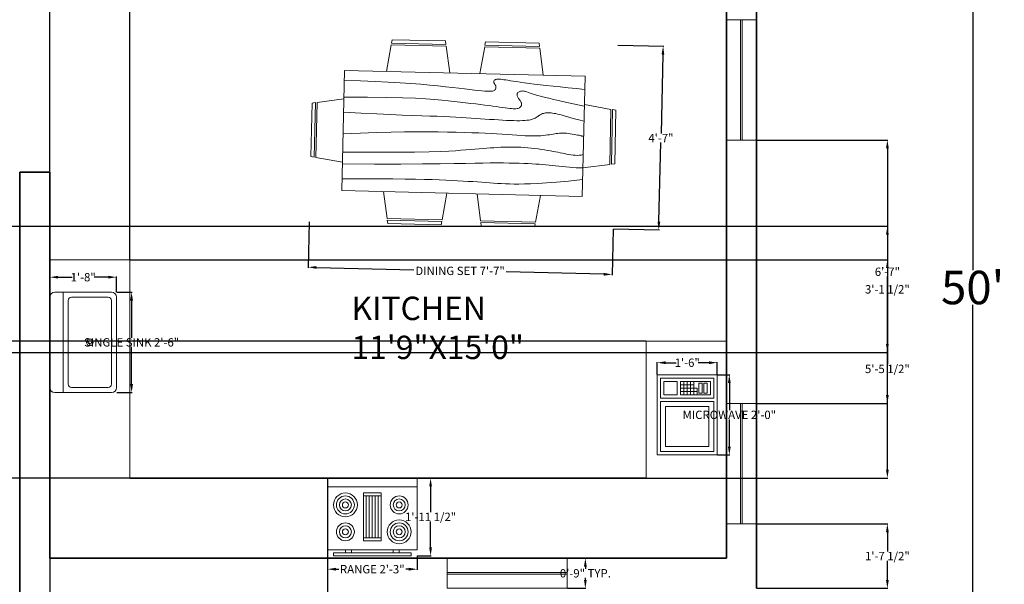
# Model space of a CAD drawing. Units: inches. Extents: x 481 to 2783, y 1975 to 3327.
# Tile 8 of 13: x 1574 to 1869, y 2866 to 3034. Entities that reach past the tile are written whole.
import ezdxf

# ---------------------------------------------------------------- set-up
doc = ezdxf.new("R2010")
doc.units = ezdxf.units.IN
doc.header["$MEASUREMENT"] = 0
for name, color, linetype, lineweight in [('A-ANNO-DIMS', 50, 'Continuous', 18), ('A-AREA-IDEN', 50, 'Continuous', 18), ('A-FLOR-CASE', 61, 'Continuous', 18), ('A-FLOR-FIXT', 61, 'Continuous', 18), ('A-FURN', 61, 'Continuous', 18), ('A-WALL', 40, 'Continuous', 35), ('EQUIPMENTS', 61, 'Continuous', 18), ('WINDOWS', 220, 'Continuous', 20)]:
    doc.layers.add(name, color=color, linetype=linetype, lineweight=lineweight)
doc.styles.get("Standard").update_dxf_attribs({"font": 'arial.ttf'})
doc.dimstyles.get("Standard").update_dxf_attribs({"dimtxt": 2.5, "dimasz": 2.5, "dimexe": 0.18, "dimexo": 0.0625, "dimgap": 0.09, "dimtad": 0, "dimtih": 1, "dimtoh": 1, "dimzin": 0, "dimdsep": 46, "dimlunit": 3, "dimtxsty": 'Standard', "dimcen": 0.09, "dimadec": 0, "dimazin": 0, "dimtfac": 1, "dimtofl": 0, "dimtmove": 0, "dimatfit": 3, "dimfxl": 1, "dimtolj": 1, "dimtzin": 0, "dimarcsym": 0})

# ---------------------------------------------------------------- blocks, each defined once
blk = doc.blocks.new('Microwave')
for p, q in [((18, 10), (22, 10)), ((22, 9), (18, 9)), ((19, 7), (19, 11)), ((20, 11), (20, 7)), ((21, 7), (21, 11)), ((18, 8), (22, 8)), ((22, 7), (18, 7)), ((20, 6), (18, 6)), ((19, 6), (19, 7)), ((20, 7), (20, 6))]:
    blk.add_line(p, q)
for points in [[(0, 0), (0, 18), (24, 18), (24, 0)], [(1, 1), (1, 17), (16, 17), (16, 1)], [(2.5, 2.5), (2.5, 15.5), (14.5, 15.5), (14.5, 2.5)], [(17, 1), (17, 17), (23, 17), (23, 1)], [(18, 12), (18, 16), (22, 16), (22, 12)], [(18, 2), (18, 11), (22, 11), (22, 2)], [(18.5, 4.5), (18.5, 5.5), (21.5, 5.5), (21.5, 4.5)], [(18.5, 3), (18.5, 4), (21.5, 4), (21.5, 3)]]:
    blk.add_lwpolyline(points, close=True)
blk = doc.blocks.new('Sink-single - 30 in top')
blk.add_line((-15, -3.999996), (15, -3.999996))
for points in [[(-13.5, 0), (13.5, 0)], [(-15, -18.499996), (-15, -1.5)], [(15, -1.5), (15, -18.499996)], [(-12.5, -5.499996), (12.5, -5.499996)], [(-13.5, -17.499996), (-13.5, -6.499996)], [(13.5, -6.499996), (13.5, -17.499996)], [(13.5, -19.999996), (-13.5, -19.999996)], [(12.5, -18.499996), (-12.5, -18.499996)]]:
    blk.add_lwpolyline(points)
for radius in [1, 0.5]:
    blk.add_circle((0, -11.999996), radius)
for centre, radius, start, end in [((-13.5, -1.5), 1.5, 90, 180), ((13.5, -1.5), 1.5, 0, 90), ((-12.5, -6.499996), 1, 90, 180), ((12.5, -6.499996), 1, 0, 90), ((-12.5, -17.499996), 1, 180, 270), ((12.5, -17.499996), 1, 270, 0), ((-13.5, -18.499996), 1.5, 180, 270), ((13.5, -18.499996), 1.5, 270, 0)]:
    blk.add_arc(centre, radius, start, end)
blk = doc.blocks.new('Dining Set - 36 x 72 in.')
for p, q in [((-22, 27.5), (-22.1562, 26.50042)), ((-22, 27.5), (-6, 27.5)), ((-5.8437, 26.49966), (-6, 27.5)), ((6, 27.5), (5.8438, 26.50042)), ((6, 27.5), (22, 27.5)), ((22.1563, 26.49966), (22, 27.5)), ((-22.2343, 26.00059), (-23.4847, 17.99762)), ((-22.2304, 26), (-5.7608, 26)), ((-5.8416, 26.5), (-22.1534, 26.5)), ((-4.5152, 17.99762), (-5.7655, 25.99926)), ((5.7657, 26.00059), (4.5153, 17.99762)), ((5.7696, 26), (22.2392, 26)), ((22.1584, 26.5), (5.8466, 26.5)), ((23.4848, 17.99762), (22.2345, 25.99926)), ((36, 18), (-36, 18)), ((-36, 18), (-36, -18)), ((36, -18), (36, 18)), ((-44.0006, 8.23428), (-35.9976, 9.48474)), ((44.0006, 8.23428), (35.9976, 9.48474)), ((-45.5, 8), (-44.5004, 8.15617)), ((-45.5, 8), (-45.5, -8)), ((-44.5, -8.15843), (-44.5, 8.15338)), ((-44, 8.23041), (-44, -8.23915)), ((44, 8.23041), (44, -8.23915)), ((44.5, -8.15843), (44.5, 8.15338)), ((45.5, 8), (44.5005, 8.15617)), ((45.5, 8), (45.5, -8)), ((-44.4997, -8.15631), (-45.5, -8)), ((-35.9976, -9.48476), (-43.9993, -8.2345)), ((35.9976, -9.48476), (43.9993, -8.2345)), ((44.4997, -8.15631), (45.5, -8)), ((-36, -18), (36, -18)), ((-22.2343, -26.0006), (-23.4847, -17.99762)), ((-4.5152, -17.99762), (-5.7655, -25.99928)), ((5.7657, -26.0006), (4.5153, -17.99762)), ((23.4848, -17.99762), (22.2345, -25.99928)), ((-22.2304, -26), (-5.7608, -26)), ((-22, -27.5), (-22.1562, -26.50044)), ((-5.8416, -26.5), (-22.1534, -26.5)), ((-5.8437, -26.49967), (-6, -27.5)), ((5.7696, -26), (22.2392, -26)), ((6, -27.5), (5.8438, -26.50044)), ((22.1584, -26.5), (5.8466, -26.5)), ((22.1563, -26.49967), (22, -27.5)), ((-22, -27.5), (-6, -27.5)), ((6, -27.5), (22, -27.5))]:
    blk.add_line(p, q)
for points in [[(-36, 15), (-31.1772, 14.97754), (-26.8079, 14.91406), (-22.8538, 14.81543), (-19.276, 14.6875), (-16.0362, 14.53613), (-13.0957, 14.36718), (-10.4159, 14.18652), (-7.9583, 14), (-5.6904, 13.81315), (-3.6035, 13.63021), (-1.6954, 13.45508), (0.0365, 13.29166), (1.5945, 13.14388), (2.9811, 13.01562), (4.1988, 12.9108), (5.25, 12.83333), (6.1393, 12.78613), (6.8802, 12.76823), (7.4883, 12.77767), (7.9792, 12.8125), (8.3685, 12.87077), (8.6719, 12.95052), (8.9049, 13.0498), (9.0833, 13.16666), (9.2205, 13.29899), (9.3216, 13.44401), (9.3895, 13.59879), (9.4271, 13.76041), (9.4373, 13.92594), (9.4232, 14.09245), (9.3875, 14.257), (9.3333, 14.41666), (9.2638, 14.56917), (9.1836, 14.71484), (9.0975, 14.85465), (9.0104, 14.98958), (8.9272, 15.1206), (8.8529, 15.2487), (8.7922, 15.37483), (8.75, 15.5), (8.7305, 15.62467), (8.7344, 15.74739), (8.7617, 15.86621), (8.8125, 15.97916), (8.8867, 16.08431), (8.9844, 16.17968), (9.1055, 16.26334), (9.25, 16.33333), (9.4189, 16.38802), (9.6172, 16.42708), (9.8506, 16.45052), (10.125, 16.45833), (10.4463, 16.45052), (10.8203, 16.42708), (11.2529, 16.38802), (11.75, 16.33333), (12.3184, 16.26318), (12.9694, 16.17838), (13.7151, 16.07991), (14.5677, 15.96875), (15.5395, 15.84586), (16.6426, 15.71224), (17.8893, 15.56884), (19.2917, 15.41666), (20.859, 15.25667), (22.5879, 15.08984), (24.4721, 14.91715), (26.5052, 14.73958), (28.6809, 14.5581), (30.9929, 14.3737), (33.4347, 14.18733), (36, 14)], [(-36, 10), (-28.9766, 10.14274), (-23.1725, 10.20442), (-18.4241, 10.19775), (-14.5677, 10.13541), (-11.4399, 10.03011), (-8.877, 9.89453), (-6.7154, 9.74137), (-4.7917, 9.58333), (-2.9698, 9.43082), (-1.2246, 9.28515), (0.4415, 9.14534), (2.026, 9.01041), (3.5266, 8.87939), (4.9408, 8.7513), (6.266, 8.62516), (7.5, 8.5), (8.6411, 8.37549), (9.6914, 8.2539), (10.6538, 8.13818), (11.5312, 8.03125), (12.3267, 7.93603), (13.043, 7.85547), (13.6831, 7.79248), (14.25, 7.75), (14.7471, 7.7303), (15.1797, 7.73307), (15.5537, 7.75732), (15.875, 7.80208), (16.1494, 7.86637), (16.3828, 7.94922), (16.5811, 8.04964), (16.75, 8.16666), (16.8944, 8.29915), (17.0143, 8.44531), (17.1089, 8.60319), (17.1771, 8.77083), (17.218, 8.94629), (17.2305, 9.1276), (17.2137, 9.31282), (17.1667, 9.5), (17.0895, 9.6875), (16.987, 9.875), (16.8649, 10.0625), (16.7292, 10.25), (16.5856, 10.4375), (16.4401, 10.625), (16.2985, 10.8125), (16.1667, 11), (16.05, 11.18733), (15.9518, 11.3737), (15.8752, 11.5581), (15.8229, 11.73958), (15.798, 11.91715), (15.8034, 12.08984), (15.842, 12.25667), (15.9167, 12.41666), (16.0295, 12.56836), (16.1784, 12.70833), (16.3605, 12.83268), (16.5729, 12.9375), (16.8127, 13.01888), (17.0768, 13.07291), (17.3625, 13.0957), (17.6667, 13.08333), (17.9894, 13.03312), (18.3418, 12.94726), (18.7382, 12.82918), (19.1927, 12.68229), (19.7195, 12.51001), (20.3327, 12.31575), (21.0465, 12.10294), (21.875, 11.875), (22.8357, 11.63354), (23.959, 11.37304), (25.2786, 11.08618), (26.8282, 10.76562), (28.6414, 10.40405), (30.752, 9.99414), (33.1936, 9.52856), (36, 9)], [(-36, 5.5), (-30.7157, 5.3348), (-26.069, 5.20963), (-21.9946, 5.11767), (-18.4271, 5.05208), (-15.3009, 5.00602), (-12.5508, 4.97265), (-10.1112, 4.94515), (-7.9167, 4.91666), (-5.909, 4.88167), (-4.0586, 4.83984), (-2.3429, 4.79215), (-0.7396, 4.73958), (0.7739, 4.6831), (2.22, 4.6237), (3.6213, 4.56233), (5, 4.5), (6.373, 4.43782), (7.7344, 4.3776), (9.0723, 4.32129), (10.375, 4.27083), (11.6309, 4.22819), (12.8281, 4.19531), (13.9551, 4.17415), (15, 4.16666), (15.954, 4.17448), (16.819, 4.19791), (17.6001, 4.23698), (18.3021, 4.29166), (18.9299, 4.36198), (19.4883, 4.44791), (19.9823, 4.54948), (20.4167, 4.66666), (20.7969, 4.79899), (21.1302, 4.94401), (21.4245, 5.09879), (21.6875, 5.26041), (21.9271, 5.42594), (22.1511, 5.59245), (22.3672, 5.757), (22.5834, 5.91666), (22.8065, 6.06868), (23.0404, 6.21093), (23.2879, 6.34147), (23.5521, 6.45833), (23.8358, 6.55957), (24.142, 6.64323), (24.4735, 6.70735), (24.8334, 6.75), (25.2235, 6.76969), (25.642, 6.76692), (26.0858, 6.74267), (26.5521, 6.69791), (27.0379, 6.63362), (27.5404, 6.55078), (28.0565, 6.45036), (28.5834, 6.33333), (29.1242, 6.19987), (29.7071, 6.04687), (30.3661, 5.87044), (31.1354, 5.66666), (32.0493, 5.43164), (33.142, 5.16146), (34.4475, 4.85221), (36, 4.5)], [(-36, -1), (-30.7915, -0.6591), (-26.0195, -0.38216), (-21.6519, -0.16284), (-17.6563, 0.00521), (-14.0005, 0.12833), (-10.6523, 0.21289), (-7.5796, 0.26522), (-4.75, 0.29166), (-2.134, 0.29793), (0.2878, 0.28711), (2.5317, 0.26163), (4.6146, 0.22396), (6.5529, 0.17651), (8.3633, 0.12174), (10.0623, 0.06209), (11.6667, 0), (13.1899, -0.06201), (14.6341, -0.1211), (15.9982, -0.17432), (17.2813, -0.21875), (18.4823, -0.25147), (19.6003, -0.26953), (20.6343, -0.27002), (21.5834, -0.25), (22.4481, -0.20768), (23.2357, -0.14584), (23.9549, -0.06836), (24.6146, 0.02083), (25.2235, 0.11784), (25.7904, 0.21875), (26.3241, 0.31966), (26.8334, 0.41666), (27.3265, 0.50618), (27.8099, 0.58593), (28.2894, 0.65397), (28.7709, 0.70833), (29.2601, 0.74707), (29.763, 0.76823), (30.2855, 0.76985), (30.8334, 0.75), (31.4088, 0.70784), (31.9994, 0.64713), (32.589, 0.57275), (33.1615, 0.48958), (33.7008, 0.4025), (34.1908, 0.3164), (34.6153, 0.23616), (34.9584, 0.16666), (35.2099, 0.11165), (35.3848, 0.07031), (35.504, 0.04069), (35.5886, 0.02083), (35.6594, 0.00879), (35.7377, 0.0026), (35.8442, 0.00032), (36, 0)], [(-36, -6.5), (-27.1843, -6.31267), (-20.084, -6.1263), (-14.469, -5.9419), (-10.1094, -5.76042), (-6.7752, -5.58285), (-4.2363, -5.41016), (-2.2629, -5.24333), (-0.625, -5.08334), (0.8708, -4.93099), (2.2715, -4.78646), (3.5872, -4.64974), (4.8281, -4.52084), (6.0046, -4.39974), (7.127, -4.28646), (8.2053, -4.18099), (9.25, -4.08334), (10.2705, -3.99382), (11.2734, -3.91407), (12.2647, -3.84603), (13.25, -3.79167), (14.2354, -3.75293), (15.2266, -3.73177), (16.2295, -3.73015), (17.25, -3.75), (18.2912, -3.79248), (19.3451, -3.85547), (20.4009, -3.93604), (21.4479, -4.03125), (22.4754, -4.13819), (23.4727, -4.25391), (24.4289, -4.37549), (25.3334, -4.5), (26.1785, -4.62492), (26.9694, -4.74935), (27.7145, -4.87281), (28.4219, -4.99479), (29.1, -5.11483), (29.7572, -5.23242), (30.4016, -5.34709), (31.0417, -5.45834), (31.6837, -5.56437), (32.3262, -5.65821), (32.9658, -5.73153), (33.599, -5.77604), (34.2224, -5.78345), (34.8327, -5.74545), (35.4264, -5.65373), (36, -5.5)], [(-36, -10), (-26.4022, -9.81299), (-18.4675, -9.62891), (-11.9839, -9.45069), (-6.7396, -9.28125), (-2.5226, -9.12354), (0.8789, -8.98047), (3.6769, -8.85498), (6.0833, -8.75), (8.2767, -8.66765), (10.3021, -8.60677), (12.1712, -8.56543), (13.8958, -8.54167), (15.4876, -8.53353), (16.9583, -8.53907), (18.3197, -8.55632), (19.5834, -8.58334), (20.7616, -8.61841), (21.8685, -8.66081), (22.9188, -8.71004), (23.9271, -8.76563), (24.9081, -8.82707), (25.8763, -8.89388), (26.8465, -8.96558), (27.8334, -9.04167), (28.8474, -9.12118), (29.8828, -9.20117), (30.93, -9.27824), (31.9792, -9.34896), (33.0205, -9.40991), (34.0443, -9.45768), (35.0407, -9.48885), (36, -9.5)], [(-36, -14.5), (-30.0881, -14.33513), (-25.0332, -14.21224), (-20.7312, -14.12647), (-17.0781, -14.07292), (-13.97, -14.04671), (-11.3027, -14.04297), (-8.9724, -14.05681), (-6.875, -14.08334), (-4.9224, -14.11833), (-3.0905, -14.16016), (-1.3709, -14.20785), (0.2448, -14.26042), (1.7647, -14.3169), (3.1973, -14.3763), (4.5507, -14.43767), (5.8333, -14.5), (7.0554, -14.5621), (8.235, -14.62175), (9.3922, -14.67652), (10.5469, -14.72396), (11.7192, -14.76164), (12.929, -14.78711), (14.1965, -14.79794), (15.5417, -14.79167), (16.9933, -14.76424), (18.6152, -14.70508), (20.4804, -14.60197), (22.6615, -14.44271), (25.2312, -14.21509), (28.2624, -13.9069), (31.8277, -13.50594), (36, -13)]]:
    blk.add_lwpolyline(points)
blk = doc.blocks.new('Range-Oven - 30 in top')
for p, q in [((0, -3), (30, -3)), ((12, -6), (18, -6)), ((13, -20), (13, -6)), ((14, -6), (14, -20)), ((15, -20), (15, -6)), ((16, -6), (16, -20)), ((17, -20), (17, -6)), ((18, -20), (12, -20)), ((6, -24), (6, -25)), ((8, -25), (8, -24)), ((22, -25), (22, -24)), ((24, -24), (24, -25))]:
    blk.add_line(p, q)
for points in [[(0, -24), (0, 0), (30, 0), (30, -24)], [(12, -21), (12, -5), (18, -5), (18, -21)], [(2, -26), (2, -25), (28, -25), (28, -26)]]:
    blk.add_lwpolyline(points, close=True)
for centre, radius in [((6, -9), 4), ((6, -9), 3), ((24, -9), 3), ((6, -9), 2), ((6, -9), 1), ((24, -9), 2), ((24, -9), 1), ((6, -18), 3), ((6, -18), 2), ((24, -18), 4), ((24, -18), 3), ((24, -18), 2), ((6, -18), 1), ((24, -18), 1)]:
    blk.add_circle(centre, radius)
blk = doc.blocks.new('*D23')
at = {"layer": 'A-ANNO-DIMS', "color": 0, "lineweight": -2, "transparency": 16777216}
for p, q in [((1794.5, 3254.32), (1859.35, 3254.32)), ((1859.17, 3249.32), (1859.17, 2959.52)), ((1859.17, 2659.32), (1859.17, 2949.13)), ((1794.5, 2654.32), (1859.35, 2654.32))]:
    blk.add_line(p, q, dxfattribs=at)
at = {"layer": 'A-ANNO-DIMS', "color": 0, "transparency": 16777216}
for points in [[(1858.33, 3249.32), (1860, 3249.32), (1859.17, 3254.32)], [(1858.33, 2659.32), (1860, 2659.32), (1859.17, 2654.32)]]:
    blk.add_solid(points, dxfattribs=at)
at = {"layer": 'Defpoints', "color": 0, "transparency": 16777216}
for p in [(1794.44, 3254.32), (1794.44, 2654.32), (1859.17, 2654.32)]:
    blk.add_point(p, dxfattribs=at)
at = {"layer": 'A-ANNO-DIMS', "color": 0, "transparency": 16777216, "insert": (1859.17, 2954.32), "char_height": 10, "attachment_point": 5}
blk.add_mtext("\\A1;50'", dxfattribs=at)
blk = doc.blocks.new('WIN-PLAN-36IN')
for p, q in [((0, 4.75), (36, 4.75)), ((0, 4.25), (36, 4.25))]:
    blk.add_line(p, q)
blk.add_lwpolyline([(0, 0), (36, 0), (36, 9), (0, 9)], close=True)
blk = doc.blocks.new('*D31')
at = {"layer": 'A-ANNO-DIMS', "color": 0, "lineweight": -2, "transparency": 16777216}
for p, q in [((1737.9, 2873.32), (1743.42, 2873.32)), ((1743.24, 2870.82), (1743.24, 2870.19)), ((1743.24, 2866.82), (1743.24, 2867.46)), ((1737.9, 2864.32), (1743.42, 2864.32))]:
    blk.add_line(p, q, dxfattribs=at)
at = {"layer": 'A-ANNO-DIMS', "color": 0, "transparency": 16777216}
for points in [[(1742.83, 2870.82), (1743.66, 2870.82), (1743.24, 2873.32)], [(1742.83, 2866.82), (1743.66, 2866.82), (1743.24, 2864.32)]]:
    blk.add_solid(points, dxfattribs=at)
at = {"layer": 'Defpoints', "color": 0, "transparency": 16777216}
for p in [(1737.84, 2873.32), (1743.24, 2873.32), (1737.84, 2864.32)]:
    blk.add_point(p, dxfattribs=at)
at = {"layer": 'A-ANNO-DIMS', "color": 0, "transparency": 16777216, "insert": (1743.24, 2868.82), "char_height": 2.5, "attachment_point": 5}
blk.add_mtext('\\A1;0\'-9" TYP.', dxfattribs=at)
blk = doc.blocks.new('*D38')
at = {"layer": 'A-ANNO-DIMS', "color": 0, "lineweight": -2, "transparency": 16777216}
for p, q in [((1782.8, 2928.23), (1786.52, 2928.23)), ((1786.34, 2925.73), (1786.34, 2917.61)), ((1786.34, 2906.73), (1786.34, 2914.84)), ((1782.8, 2904.23), (1786.52, 2904.23))]:
    blk.add_line(p, q, dxfattribs=at)
at = {"layer": 'A-ANNO-DIMS', "color": 0, "transparency": 16777216}
for points in [[(1785.92, 2925.73), (1786.76, 2925.73), (1786.34, 2928.23)], [(1785.92, 2906.73), (1786.76, 2906.73), (1786.34, 2904.23)]]:
    blk.add_solid(points, dxfattribs=at)
at = {"layer": 'Defpoints', "color": 0, "transparency": 16777216}
for p in [(1782.74, 2928.23), (1786.34, 2928.23), (1782.74, 2904.23)]:
    blk.add_point(p, dxfattribs=at)
at = {"layer": 'A-ANNO-DIMS', "color": 0, "transparency": 16777216, "insert": (1786.34, 2916.23), "char_height": 2.5, "attachment_point": 5}
blk.add_mtext('\\A1;MICROWAVE 2\'-0"', dxfattribs=at)
blk = doc.blocks.new('*D39')
at = {"layer": 'A-ANNO-DIMS', "color": 0, "lineweight": -2, "transparency": 16777216}
for p, q in [((1764.74, 2928.29), (1764.74, 2932.01)), ((1767.24, 2931.83), (1770.45, 2931.83)), ((1780.24, 2931.83), (1777.04, 2931.83)), ((1782.74, 2928.29), (1782.74, 2932.01))]:
    blk.add_line(p, q, dxfattribs=at)
at = {"layer": 'A-ANNO-DIMS', "color": 0, "transparency": 16777216}
for points in [[(1767.24, 2932.24), (1767.24, 2931.41), (1764.74, 2931.83)], [(1780.24, 2932.24), (1780.24, 2931.41), (1782.74, 2931.83)]]:
    blk.add_solid(points, dxfattribs=at)
at = {"layer": 'Defpoints', "color": 0, "transparency": 16777216}
for p in [(1764.74, 2931.83), (1764.74, 2928.23), (1782.74, 2928.23)]:
    blk.add_point(p, dxfattribs=at)
at = {"layer": 'A-ANNO-DIMS', "color": 0, "transparency": 16777216, "insert": (1773.74, 2931.83), "char_height": 2.5, "attachment_point": 5}
blk.add_mtext('\\A1;1\'-6"', dxfattribs=at)
blk = doc.blocks.new('*D42')
at = {"layer": 'A-ANNO-DIMS', "color": 0, "lineweight": -2, "transparency": 16777216}
for p, q in [((1603, 2952.91), (1607.62, 2952.91)), ((1607.44, 2950.41), (1607.44, 2939.29)), ((1607.44, 2925.41), (1607.44, 2936.53)), ((1603, 2922.91), (1607.62, 2922.91))]:
    blk.add_line(p, q, dxfattribs=at)
at = {"layer": 'A-ANNO-DIMS', "color": 0, "transparency": 16777216}
for points in [[(1607.02, 2950.41), (1607.85, 2950.41), (1607.44, 2952.91)], [(1607.02, 2925.41), (1607.85, 2925.41), (1607.44, 2922.91)]]:
    blk.add_solid(points, dxfattribs=at)
at = {"layer": 'Defpoints', "color": 0, "transparency": 16777216}
for p in [(1602.94, 2952.91), (1607.44, 2952.91), (1602.94, 2922.91)]:
    blk.add_point(p, dxfattribs=at)
at = {"layer": 'A-ANNO-DIMS', "color": 0, "transparency": 16777216, "insert": (1607.44, 2937.91), "char_height": 2.5, "attachment_point": 5}
blk.add_mtext('\\A1;SINGLE SINK 2\'-6"', dxfattribs=at)
blk = doc.blocks.new('*D43')
at = {"layer": 'A-ANNO-DIMS', "color": 0, "lineweight": -2, "transparency": 16777216}
for p, q in [((1582.94, 2952.97), (1582.94, 2957.59)), ((1585.44, 2957.41), (1589.64, 2957.41)), ((1600.44, 2957.41), (1596.23, 2957.41)), ((1602.94, 2952.97), (1602.94, 2957.59))]:
    blk.add_line(p, q, dxfattribs=at)
at = {"layer": 'A-ANNO-DIMS', "color": 0, "transparency": 16777216}
for points in [[(1585.44, 2957.83), (1585.44, 2956.99), (1582.94, 2957.41)], [(1600.44, 2957.83), (1600.44, 2956.99), (1602.94, 2957.41)]]:
    blk.add_solid(points, dxfattribs=at)
at = {"layer": 'Defpoints', "color": 0, "transparency": 16777216}
for p in [(1582.94, 2957.41), (1582.94, 2952.91), (1602.94, 2952.91)]:
    blk.add_point(p, dxfattribs=at)
at = {"layer": 'A-ANNO-DIMS', "color": 0, "transparency": 16777216, "insert": (1592.94, 2957.41), "char_height": 2.5, "attachment_point": 5}
blk.add_mtext('\\A1;1\'-8"', dxfattribs=at)
blk = doc.blocks.new('*D50')
at = {"layer": 'A-ANNO-DIMS', "color": 0, "lineweight": -2, "transparency": 16777216}
for p, q in [((1660.59, 2973.97), (1660.26, 2960.21)), ((1751.56, 2971.8), (1751.23, 2958.04)), ((1662.76, 2960.33), (1691.92, 2959.63)), ((1748.74, 2958.28), (1719.58, 2958.98))]:
    blk.add_line(p, q, dxfattribs=at)
at = {"layer": 'A-ANNO-DIMS', "color": 0, "transparency": 16777216}
for points in [[(1662.77, 2960.74), (1662.75, 2959.91), (1660.26, 2960.39)], [(1748.75, 2958.7), (1748.73, 2957.86), (1751.24, 2958.22)]]:
    blk.add_solid(points, dxfattribs=at)
at = {"layer": 'Defpoints', "color": 0, "transparency": 16777216}
for p in [(1660.59, 2974.03), (1751.56, 2971.87), (1751.24, 2958.22)]:
    blk.add_point(p, dxfattribs=at)
at = {"layer": 'A-ANNO-DIMS', "color": 0, "transparency": 16777216, "insert": (1705.75, 2959.3), "char_height": 2.5, "attachment_point": 5}
blk.add_mtext('\\A1;DINING SET 7\'-7"', dxfattribs=at)
blk = doc.blocks.new('*D51')
at = {"layer": 'A-ANNO-DIMS', "color": 0, "lineweight": -2, "transparency": 16777216}
for p, q in [((1752.93, 3026.85), (1766.7, 3026.52)), ((1766.46, 3024.03), (1765.89, 3000.37)), ((1765.27, 2974.04), (1765.83, 2997.69)), ((1751.62, 2971.87), (1765.39, 2971.54))]:
    blk.add_line(p, q, dxfattribs=at)
at = {"layer": 'A-ANNO-DIMS', "color": 0, "transparency": 16777216}
for points in [[(1766.04, 3024.04), (1766.87, 3024.02), (1766.52, 3026.53)], [(1764.85, 2974.05), (1765.68, 2974.03), (1765.21, 2971.54)]]:
    blk.add_solid(points, dxfattribs=at)
at = {"layer": 'Defpoints', "color": 0, "transparency": 16777216}
for p in [(1752.87, 3026.85), (1766.52, 3026.53), (1751.56, 2971.87)]:
    blk.add_point(p, dxfattribs=at)
at = {"layer": 'A-ANNO-DIMS', "color": 0, "transparency": 16777216, "insert": (1765.86, 2999.03), "char_height": 2.5, "attachment_point": 5}
blk.add_mtext('\\A1;4\'-7"', dxfattribs=at)
blk = doc.blocks.new('*D52')
at = {"layer": 'A-ANNO-DIMS', "color": 0, "lineweight": -2, "transparency": 16777216}
for p, q in [((1666.06, 2874.01), (1666.06, 2869.86)), ((1692.89, 2874.01), (1692.89, 2869.86)), ((1668.56, 2870.04), (1669.43, 2870.04)), ((1690.39, 2870.04), (1689.52, 2870.04))]:
    blk.add_line(p, q, dxfattribs=at)
at = {"layer": 'A-ANNO-DIMS', "color": 0, "transparency": 16777216}
for points in [[(1668.56, 2870.46), (1668.56, 2869.63), (1666.06, 2870.04)], [(1690.39, 2870.46), (1690.39, 2869.63), (1692.89, 2870.04)]]:
    blk.add_solid(points, dxfattribs=at)
at = {"layer": 'Defpoints', "color": 0, "transparency": 16777216}
for p in [(1666.06, 2874.07), (1692.89, 2874.07), (1692.89, 2870.04)]:
    blk.add_point(p, dxfattribs=at)
at = {"layer": 'A-ANNO-DIMS', "color": 0, "transparency": 16777216, "insert": (1679.47, 2870.04), "char_height": 2.5, "attachment_point": 5}
blk.add_mtext('\\A1;RANGE 2\'-3"', dxfattribs=at)
blk = doc.blocks.new('*D53')
at = {"layer": 'A-ANNO-DIMS', "color": 0, "lineweight": -2, "transparency": 16777216}
for p, q in [((1692.95, 2897.32), (1697.1, 2897.32)), ((1696.92, 2894.82), (1696.92, 2887.08)), ((1696.92, 2876.57), (1696.92, 2884.31)), ((1692.95, 2874.07), (1697.1, 2874.07))]:
    blk.add_line(p, q, dxfattribs=at)
at = {"layer": 'A-ANNO-DIMS', "color": 0, "transparency": 16777216}
for points in [[(1696.5, 2894.82), (1697.33, 2894.82), (1696.92, 2897.32)], [(1696.5, 2876.57), (1697.33, 2876.57), (1696.92, 2874.07)]]:
    blk.add_solid(points, dxfattribs=at)
at = {"layer": 'Defpoints', "color": 0, "transparency": 16777216}
for p in [(1692.89, 2897.32), (1696.92, 2897.32), (1692.89, 2874.07)]:
    blk.add_point(p, dxfattribs=at)
at = {"layer": 'A-ANNO-DIMS', "color": 0, "transparency": 16777216, "insert": (1696.92, 2885.7), "char_height": 2.5, "attachment_point": 5}
blk.add_mtext('\\A1;1\'-11 1/2"', dxfattribs=at)
blk = doc.blocks.new('*D88')
at = {"layer": 'A-ANNO-DIMS', "color": 0, "lineweight": -2, "transparency": 16777216}
for p, q in [((1794.5, 2883.62), (1833.82, 2883.62)), ((1833.64, 2881.12), (1833.64, 2875.35)), ((1833.64, 2866.82), (1833.64, 2872.59)), ((1794.5, 2864.32), (1833.82, 2864.32))]:
    blk.add_line(p, q, dxfattribs=at)
at = {"layer": 'A-ANNO-DIMS', "color": 0, "transparency": 16777216}
for points in [[(1833.22, 2881.12), (1834.05, 2881.12), (1833.64, 2883.62)], [(1833.22, 2866.82), (1834.05, 2866.82), (1833.64, 2864.32)]]:
    blk.add_solid(points, dxfattribs=at)
at = {"layer": 'Defpoints', "color": 0, "transparency": 16777216}
for p in [(1794.44, 2883.62), (1833.64, 2883.62), (1794.44, 2864.32)]:
    blk.add_point(p, dxfattribs=at)
at = {"layer": 'A-ANNO-DIMS', "color": 0, "transparency": 16777216, "insert": (1833.64, 2873.97), "char_height": 2.5, "attachment_point": 5}
blk.add_mtext('\\A1;1\'-7 1/2"', dxfattribs=at)
blk = doc.blocks.new('*D89')
at = {"layer": 'A-ANNO-DIMS', "color": 0, "lineweight": -2, "transparency": 16777216}
for p, q in [((1794.5, 2998.45), (1833.82, 2998.45)), ((1833.64, 2995.95), (1833.64, 2960.4)), ((1833.64, 2922.12), (1833.64, 2957.67)), ((1794.5, 2919.62), (1833.82, 2919.62))]:
    blk.add_line(p, q, dxfattribs=at)
at = {"layer": 'A-ANNO-DIMS', "color": 0, "transparency": 16777216}
for points in [[(1833.22, 2995.95), (1834.05, 2995.95), (1833.64, 2998.45)], [(1833.22, 2922.12), (1834.05, 2922.12), (1833.64, 2919.62)]]:
    blk.add_solid(points, dxfattribs=at)
at = {"layer": 'Defpoints', "color": 0, "transparency": 16777216}
for p in [(1794.44, 2998.45), (1833.64, 2998.45), (1794.44, 2919.62)]:
    blk.add_point(p, dxfattribs=at)
at = {"layer": 'A-ANNO-DIMS', "color": 0, "transparency": 16777216, "insert": (1833.64, 2959.03), "char_height": 2.5, "attachment_point": 5}
blk.add_mtext('\\A1;6\'-7"', dxfattribs=at)
blk = doc.blocks.new('*D97')
at = {"layer": 'A-ANNO-DIMS', "color": 0, "lineweight": -2, "transparency": 16777216}
for p, q in [((1520, 2972.64), (1833.82, 2972.64)), ((1833.64, 2970.14), (1833.64, 2955.16)), ((1833.64, 2937.42), (1833.64, 2952.39)), ((1520, 2934.92), (1833.82, 2934.92))]:
    blk.add_line(p, q, dxfattribs=at)
at = {"layer": 'A-ANNO-DIMS', "color": 0, "transparency": 16777216}
for points in [[(1833.22, 2970.14), (1834.05, 2970.14), (1833.64, 2972.64)], [(1833.22, 2937.42), (1834.05, 2937.42), (1833.64, 2934.92)]]:
    blk.add_solid(points, dxfattribs=at)
at = {"layer": 'Defpoints', "color": 0, "transparency": 16777216}
for p in [(1519.94, 2972.64), (1833.64, 2972.64), (1519.94, 2934.92)]:
    blk.add_point(p, dxfattribs=at)
at = {"layer": 'A-ANNO-DIMS', "color": 0, "transparency": 16777216, "insert": (1833.64, 2953.78), "char_height": 2.5, "attachment_point": 5}
blk.add_mtext('\\A1;3\'-1 1/2"', dxfattribs=at)
blk = doc.blocks.new('*D101')
at = {"layer": 'A-ANNO-DIMS', "color": 0, "lineweight": -2, "transparency": 16777216}
for p, q in [((1582.94, 2962.67), (1582.94, 3293.7)), ((1585.44, 3293.52), (1591.5, 3293.52)), ((1604.44, 3293.52), (1598.37, 3293.52)), ((1606.94, 2962.67), (1606.94, 3293.7))]:
    blk.add_line(p, q, dxfattribs=at)
at = {"layer": 'A-ANNO-DIMS', "color": 0, "transparency": 16777216}
for points in [[(1585.44, 3293.94), (1585.44, 3293.11), (1582.94, 3293.52)], [(1604.44, 3293.94), (1604.44, 3293.11), (1606.94, 3293.52)]]:
    blk.add_solid(points, dxfattribs=at)
at = {"layer": 'Defpoints', "color": 0, "transparency": 16777216}
for p in [(1606.94, 3293.52), (1582.94, 2962.61), (1606.94, 2962.61)]:
    blk.add_point(p, dxfattribs=at)
at = {"layer": 'A-ANNO-DIMS', "color": 0, "transparency": 16777216, "insert": (1594.94, 3293.52), "char_height": 2.5, "attachment_point": 5}
blk.add_mtext('\\A1;2\'-0"', dxfattribs=at)
blk = doc.blocks.new('*D102')
at = {"layer": 'A-ANNO-DIMS', "color": 0, "lineweight": -2, "transparency": 16777216}
for p, q in [((1607, 2962.61), (1833.82, 2962.61)), ((1833.64, 2960.11), (1833.64, 2931.35)), ((1833.64, 2899.82), (1833.64, 2928.58)), ((1607, 2897.32), (1833.82, 2897.32))]:
    blk.add_line(p, q, dxfattribs=at)
at = {"layer": 'A-ANNO-DIMS', "color": 0, "transparency": 16777216}
for points in [[(1833.22, 2960.11), (1834.05, 2960.11), (1833.64, 2962.61)], [(1833.22, 2899.82), (1834.05, 2899.82), (1833.64, 2897.32)]]:
    blk.add_solid(points, dxfattribs=at)
at = {"layer": 'Defpoints', "color": 0, "transparency": 16777216}
for p in [(1606.94, 2962.61), (1606.94, 2897.32), (1833.64, 2897.32)]:
    blk.add_point(p, dxfattribs=at)
at = {"layer": 'A-ANNO-DIMS', "color": 0, "transparency": 16777216, "insert": (1833.64, 2929.97), "char_height": 2.5, "attachment_point": 5}
blk.add_mtext('\\A1;5\'-5 1/2"', dxfattribs=at)
blk = doc.blocks.new('*D103')
at = {"layer": 'A-ANNO-DIMS', "color": 0, "lineweight": -2, "transparency": 16777216}
for p, q in [((1761.38, 2938.3), (1335.06, 2938.3)), ((1335.24, 2935.8), (1335.24, 2919.18)), ((1335.24, 2899.82), (1335.24, 2916.45)), ((1761.38, 2897.32), (1335.06, 2897.32))]:
    blk.add_line(p, q, dxfattribs=at)
at = {"layer": 'A-ANNO-DIMS', "color": 0, "transparency": 16777216}
for points in [[(1334.82, 2935.8), (1335.65, 2935.8), (1335.24, 2938.3)], [(1334.82, 2899.82), (1335.65, 2899.82), (1335.24, 2897.32)]]:
    blk.add_solid(points, dxfattribs=at)
at = {"layer": 'Defpoints', "color": 0, "transparency": 16777216}
for p in [(1335.24, 2938.3), (1761.44, 2938.3), (1761.44, 2897.32)]:
    blk.add_point(p, dxfattribs=at)
at = {"layer": 'A-ANNO-DIMS', "color": 0, "transparency": 16777216, "insert": (1335.24, 2917.81), "char_height": 2.5, "attachment_point": 5}
blk.add_mtext('\\A1;3\'-5"', dxfattribs=at)
blk = doc.blocks.new('*D104')
at = {"layer": 'A-ANNO-DIMS', "color": 0, "lineweight": -2, "transparency": 16777216}
for p, q in [((1666.06, 2897.26), (1666.06, 2614.94)), ((1582.94, 2873.26), (1582.94, 2614.94)), ((1585.44, 2615.12), (1620.11, 2615.12)), ((1663.56, 2615.12), (1628.89, 2615.12))]:
    blk.add_line(p, q, dxfattribs=at)
at = {"layer": 'A-ANNO-DIMS', "color": 0, "transparency": 16777216}
for points in [[(1585.44, 2615.54), (1585.44, 2614.71), (1582.94, 2615.12)], [(1663.56, 2615.54), (1663.56, 2614.71), (1666.06, 2615.12)]]:
    blk.add_solid(points, dxfattribs=at)
at = {"layer": 'Defpoints', "color": 0, "transparency": 16777216}
for p in [(1666.06, 2897.32), (1582.94, 2873.32), (1666.06, 2615.12)]:
    blk.add_point(p, dxfattribs=at)
at = {"layer": 'A-ANNO-DIMS', "color": 0, "transparency": 16777216, "insert": (1624.5, 2615.12), "char_height": 2.5, "attachment_point": 5}
blk.add_mtext('\\A1;6\'-11"', dxfattribs=at)

msp = doc.modelspace()

# ---------------------------------------------------------------- linework, layer by layer
at = {"layer": 'A-FLOR-CASE'}
for p, q in [((1582.938, 2962.607), (1606.938, 2962.607)), ((1606.938, 2962.607), (1606.938, 2897.323)), ((1761.438, 2897.323), (1761.438, 2938.303)), ((1761.438, 2938.303), (1785.438, 2938.303)), ((1761.438, 2897.323), (1606.938, 2897.323))]:
    msp.add_line(p, q, dxfattribs=at)
at = {"layer": 'A-WALL'}
for p, q in [((1785.438, 2873.323), (1785.438, 3053.323)), ((1582.938, 2988.823), (1573.938, 2988.823)), ((1573.938, 2988.823), (1573.938, 2808.823)), ((1582.938, 2988.823), (1582.938, 2873.323)), ((1785.438, 2873.323), (1582.938, 2873.323))]:
    msp.add_line(p, q, dxfattribs=at)
msp.add_lwpolyline([(1794.438, 2864.323), (1794.438, 3254.323), (1374.438, 3254.323), (1374.438, 2654.323), (1582.938, 2654.323)], dxfattribs=at)

# ---------------------------------------------------------------- block references
at = {"layer": 'A-FLOR-FIXT', "rotation": 90}
msp.add_blockref('Sink-single - 30 in top', (1582.938, 2937.911), dxfattribs=at)
at = {"layer": 'A-FURN', "rotation": 358.6359524520812}
msp.add_blockref('Dining Set - 36 x 72 in.', (1706.729, 3000.443), dxfattribs=at)
at = {"layer": 'EQUIPMENTS', "rotation": 90}
msp.add_blockref('Microwave', (1782.74, 2904.226), dxfattribs=at)
at = {"layer": 'EQUIPMENTS', "xscale": 0.8944269405603023, "yscale": 0.8944269405603023, "zscale": 0.8944269405603023}
msp.add_blockref('Range-Oven - 30 in top', (1666.058, 2897.323), dxfattribs=at)
at = {"layer": 'WINDOWS'}
for p, rotation in [((1794.438, 2998.448), 90.0000000000003), ((1794.438, 2883.616), 89.99999999999909)]:
    msp.add_blockref('WIN-PLAN-36IN', p, dxfattribs=dict(at, rotation=rotation))
msp.add_blockref('WIN-PLAN-36IN', (1701.842, 2864.323), dxfattribs=at)

# ---------------------------------------------------------------- texts
at = {"layer": 'A-AREA-IDEN', "insert": (1673.237, 2951.584), "char_height": 7, "attachment_point": 1}
msp.add_mtext_dynamic_manual_height_columns('KITCHEN\\P11\'9"X15\'0"', width=43.33543, gutter_width=1, heights=[0], dxfattribs=at)

# ---------------------------------------------------------------- dimensions: what is measured, and where the dimension line sits
at = {"layer": 'A-ANNO-DIMS'}
for base, p1, p2, picture, middle in [((1606.938, 3293.523), (1582.938, 2962.607), (1606.938, 2962.607), '*D101', (1594.938, 3293.523)), ((1666.058, 2615.123), (1582.938, 2873.323), (1666.058, 2897.323), '*D104', (1624.498, 2615.123))]:
    dim = msp.add_linear_dim(base=base, p1=p1, p2=p2, dimstyle='Standard', override={"dimdec": 1, "dimlfac": 1, "dimrnd": 0, "dimzin": 1, "dimdsep": 46, "dimlunit": 4, "dimfrac": 2}, dxfattribs=at)
    dim.commit()
    dim.dimension.update_dxf_attribs({"geometry": picture, "text_midpoint": middle})
dim = msp.add_aligned_dim(p1=(1794.438, 3254.323), p2=(1794.438, 2654.323), distance=64.73, dimstyle='Standard', override={"dimtxt": 10, "dimasz": 5, "dimclrd": 0, "dimclre": 0, "dimclrt": 0}, dxfattribs=at)
dim.commit()
dim.dimension.update_dxf_attribs({"geometry": '*D23', "text_midpoint": (1859.168, 2954.323)})
for base, p1, p2, angle, picture, middle in [((1766.517, 3026.527), (1751.562, 2971.867), (1752.871, 3026.852), 88.63595, '*D51', (1765.862, 2999.035)), ((1833.638, 2998.448), (1794.438, 2919.616), (1794.438, 2998.448), 90, '*D89', (1833.638, 2959.032)), ((1833.638, 2972.637), (1519.938, 2934.918), (1519.938, 2972.637), 90, '*D97', (1833.638, 2953.778)), ((1833.638, 2897.323), (1606.938, 2962.607), (1606.938, 2897.323), 90, '*D102', (1833.638, 2929.965)), ((1582.938, 2957.411), (1602.938, 2952.911), (1582.938, 2952.911), 180, '*D43', (1592.938, 2957.411)), ((1335.238, 2938.303), (1761.438, 2897.323), (1761.438, 2938.303), 90, '*D103', (1335.238, 2917.813)), ((1764.74, 2931.826), (1782.74, 2928.226), (1764.74, 2928.226), 180, '*D39', (1773.74, 2931.826)), ((1696.916, 2897.323), (1692.891, 2874.068), (1692.891, 2897.323), 90, '*D53', (1696.916, 2885.695)), ((1833.638, 2883.616), (1794.438, 2864.323), (1794.438, 2883.616), 90, '*D88', (1833.638, 2873.97))]:
    dim = msp.add_linear_dim(base=base, p1=p1, p2=p2, angle=angle, dimstyle='Standard', override={"dimdec": 1, "dimlfac": 1, "dimrnd": 0, "dimzin": 1, "dimdsep": 46, "dimlunit": 4, "dimfrac": 2}, dxfattribs=at)
    dim.commit()
    dim.dimension.update_dxf_attribs({"geometry": picture, "text_midpoint": middle})
for base, p1, p2, angle, text, picture, middle in [((1751.237, 2958.221), (1660.587, 2974.034), (1751.562, 2971.867), 358.63595, 'DINING SET <>', '*D50', (1705.75, 2959.304)), ((1607.438, 2952.911), (1602.938, 2922.911), (1602.938, 2952.911), 90, 'SINGLE SINK <>', '*D42', (1607.438, 2937.911)), ((1786.34, 2928.226), (1782.74, 2904.226), (1782.74, 2928.226), 90, 'MICROWAVE <>', '*D38', (1786.34, 2916.226)), ((1743.242, 2873.323), (1737.842, 2864.323), (1737.842, 2873.323), 90, '<> TYP.', '*D31', (1743.242, 2868.823))]:
    dim = msp.add_linear_dim(base=base, p1=p1, p2=p2, angle=angle, text=text, dimstyle='Standard', override={"dimdec": 1, "dimlfac": 1, "dimrnd": 0, "dimzin": 1, "dimdsep": 46, "dimlunit": 4, "dimfrac": 2}, dxfattribs=at)
    dim.commit()
    dim.dimension.update_dxf_attribs({"geometry": picture, "text_midpoint": middle})
dim = msp.add_linear_dim(base=(1692.891, 2870.043), p1=(1666.058, 2874.068), p2=(1692.891, 2874.068), text='RANGE <>', dimstyle='Standard', override={"dimdec": 1, "dimlfac": 1, "dimrnd": 0, "dimzin": 1, "dimdsep": 46, "dimlunit": 4, "dimfrac": 2}, dxfattribs=at)
dim.commit()
dim.dimension.update_dxf_attribs({"geometry": '*D52', "text_midpoint": (1679.475, 2870.043)})

doc.saveas('drawing.dxf')
